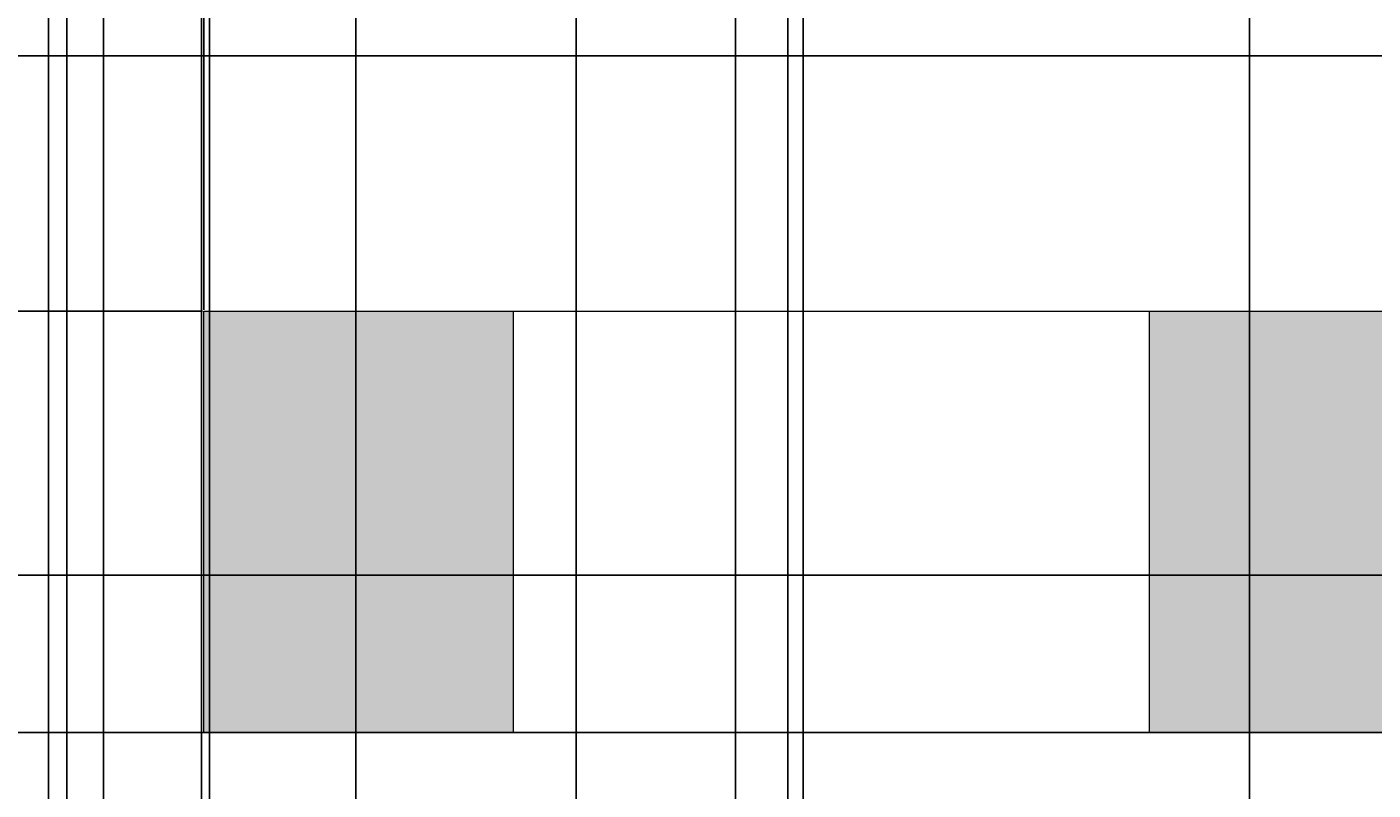
# Model space of a CAD drawing. Units: inches. Extents: x 818 to 1898, y 976 to 2364.
# Tile 68 of 96: x 1302 to 1372, y 1873 to 1913. Entities that reach past the tile are written whole.
import ezdxf

# ---------------------------------------------------------------- set-up
doc = ezdxf.new("R2010")
doc.units = ezdxf.units.IN
doc.header["$LTSCALE"] = 5
doc.header["$MEASUREMENT"] = 0
for name, color, linetype, lineweight in [('A-ANNO-DIMS', 2, 'Continuous', 18), ('A-FLOR-CASE', 8, 'Continuous', 18), ('A-FURN-PATT', 8, 'Continuous', 9)]:
    doc.layers.add(name, color=color, linetype=linetype, lineweight=lineweight)
doc.styles.get("Standard").update_dxf_attribs({"font": 'arial.ttf'})
doc.dimstyles.get("Standard").update_dxf_attribs({"dimtxt": 0.18, "dimasz": 0.18, "dimexe": 0.18, "dimexo": 0.0625, "dimgap": 0.09, "dimtad": 0, "dimtih": 1, "dimtoh": 1, "dimdec": 4, "dimzin": 0, "dimdsep": 46, "dimtxsty": 'Standard', "dimcen": 0.09, "dimadec": 0, "dimazin": 0, "dimtfac": 1, "dimtdec": 4, "dimtofl": 0, "dimtmove": 0, "dimatfit": 3, "dimfxl": 1, "dimtolj": 1, "dimtzin": 0, "dimarcsym": 0})

# ---------------------------------------------------------------- blocks, each defined once
blk = doc.blocks.new('*D61')
at = {"layer": 'A-ANNO-DIMS', "color": 0, "lineweight": -2, "ltscale": 5, "transparency": 16777216}
for p, q in [((1071.725, 1203.027), (1071.725, 2363.873)), ((1071.905, 2363.693), (1250.936, 2363.693)), ((1430.545, 2363.693), (1251.514, 2363.693)), ((1430.725, 1203.027), (1430.725, 2363.873))]:
    blk.add_line(p, q, dxfattribs=at)
at = {"layer": 'A-ANNO-DIMS', "color": 0, "ltscale": 5, "transparency": 16777216}
for points in [[(1071.905, 2363.723), (1071.905, 2363.663), (1071.725, 2363.693)], [(1430.545, 2363.723), (1430.545, 2363.663), (1430.725, 2363.693)]]:
    blk.add_solid(points, dxfattribs=at)
at = {"layer": 'Defpoints', "color": 0, "ltscale": 5, "transparency": 16777216}
for p in [(1430.725, 2363.693), (1071.725, 1202.964), (1430.725, 1202.964)]:
    blk.add_point(p, dxfattribs=at)
at = {"layer": 'A-ANNO-DIMS', "color": 0, "ltscale": 5, "transparency": 16777216, "insert": (1251.225, 2363.693), "char_height": 0.18, "attachment_point": 5}
blk.add_mtext('\\A1;359', dxfattribs=at)
blk = doc.blocks.new('*D64')
at = {"layer": 'A-ANNO-DIMS', "color": 0, "lineweight": -2, "ltscale": 5, "transparency": 16777216}
for p, q in [((1197.725, 1501.141), (1197.725, 2363.873)), ((1197.905, 2363.693), (1313.935, 2363.693)), ((1430.545, 2363.693), (1314.516, 2363.693)), ((1430.725, 1501.141), (1430.725, 2363.873))]:
    blk.add_line(p, q, dxfattribs=at)
at = {"layer": 'A-ANNO-DIMS', "color": 0, "ltscale": 5, "transparency": 16777216}
for points in [[(1197.905, 2363.723), (1197.905, 2363.663), (1197.725, 2363.693)], [(1430.545, 2363.723), (1430.545, 2363.663), (1430.725, 2363.693)]]:
    blk.add_solid(points, dxfattribs=at)
at = {"layer": 'Defpoints', "color": 0, "ltscale": 5, "transparency": 16777216}
for p in [(1430.725, 2363.693), (1197.725, 1501.078), (1430.725, 1501.078)]:
    blk.add_point(p, dxfattribs=at)
at = {"layer": 'A-ANNO-DIMS', "color": 0, "ltscale": 5, "transparency": 16777216, "insert": (1314.225, 2363.693), "char_height": 0.18, "attachment_point": 5}
blk.add_mtext('\\A1;233', dxfattribs=at)
blk = doc.blocks.new('*D74')
at = {"layer": 'A-ANNO-DIMS', "color": 0, "lineweight": -2, "ltscale": 5, "transparency": 16777216}
for p, q in [((1590.663, 1940.078), (818.026, 1940.078)), ((818.206, 1939.898), (818.206, 1925.76)), ((818.206, 1911.258), (818.206, 1925.396)), ((1590.663, 1911.078), (818.026, 1911.078))]:
    blk.add_line(p, q, dxfattribs=at)
at = {"layer": 'A-ANNO-DIMS', "color": 0, "ltscale": 5, "transparency": 16777216}
for points in [[(818.176, 1939.898), (818.236, 1939.898), (818.206, 1940.078)], [(818.176, 1911.258), (818.236, 1911.258), (818.206, 1911.078)]]:
    blk.add_solid(points, dxfattribs=at)
at = {"layer": 'Defpoints', "color": 0, "ltscale": 5, "transparency": 16777216}
for p in [(818.206, 1940.078), (1590.725, 1940.078), (1590.725, 1911.078)]:
    blk.add_point(p, dxfattribs=at)
at = {"layer": 'A-ANNO-DIMS', "color": 0, "ltscale": 5, "transparency": 16777216, "insert": (818.206, 1925.578), "char_height": 0.18, "attachment_point": 5}
blk.add_mtext('\\A1;29', dxfattribs=at)
blk = doc.blocks.new('*D85')
at = {"layer": 'A-ANNO-DIMS', "color": 0, "lineweight": -2, "ltscale": 5, "transparency": 16777216}
for p, q in [((1258.788, 2053.078), (1897.916, 2053.078)), ((1897.736, 2052.898), (1897.736, 1876.76)), ((1897.736, 1700.258), (1897.736, 1876.396)), ((1258.788, 1700.078), (1897.916, 1700.078))]:
    blk.add_line(p, q, dxfattribs=at)
at = {"layer": 'A-ANNO-DIMS', "color": 0, "ltscale": 5, "transparency": 16777216}
for points in [[(1897.706, 2052.898), (1897.766, 2052.898), (1897.736, 2053.078)], [(1897.706, 1700.258), (1897.766, 1700.258), (1897.736, 1700.078)]]:
    blk.add_solid(points, dxfattribs=at)
at = {"layer": 'Defpoints', "color": 0, "ltscale": 5, "transparency": 16777216}
for p in [(1258.725, 2053.078), (1897.736, 2053.078), (1258.725, 1700.078)]:
    blk.add_point(p, dxfattribs=at)
at = {"layer": 'A-ANNO-DIMS', "color": 0, "ltscale": 5, "transparency": 16777216, "insert": (1897.736, 1876.578), "char_height": 0.18, "attachment_point": 5}
blk.add_mtext('\\A1;353', dxfattribs=at)
blk = doc.blocks.new('*D97')
at = {"layer": 'A-ANNO-DIMS', "color": 0, "lineweight": -2, "ltscale": 5, "transparency": 16777216}
for p, q in [((1284.17, 1071.118), (1284.17, 2363.873)), ((1284.35, 2363.693), (1310.962, 2363.693)), ((1338.361, 2363.693), (1311.749, 2363.693)), ((1338.541, 1071.118), (1338.541, 2363.873))]:
    blk.add_line(p, q, dxfattribs=at)
at = {"layer": 'A-ANNO-DIMS', "color": 0, "ltscale": 5, "transparency": 16777216}
for points in [[(1284.35, 2363.723), (1284.35, 2363.663), (1284.17, 2363.693)], [(1338.361, 2363.723), (1338.361, 2363.663), (1338.541, 2363.693)]]:
    blk.add_solid(points, dxfattribs=at)
at = {"layer": 'Defpoints', "color": 0, "ltscale": 5, "transparency": 16777216}
for p in [(1338.541, 2363.693), (1284.17, 1071.055), (1338.541, 1071.055)]:
    blk.add_point(p, dxfattribs=at)
at = {"layer": 'A-ANNO-DIMS', "color": 0, "ltscale": 5, "transparency": 16777216, "insert": (1311.355, 2363.693), "char_height": 0.18, "attachment_point": 5}
blk.add_mtext('\\A1;54.37', dxfattribs=at)
blk = doc.blocks.new('*D98')
at = {"layer": 'A-ANNO-DIMS', "color": 0, "lineweight": -2, "ltscale": 5, "transparency": 16777216}
for p, q in [((1338.541, 1071.118), (1338.541, 2363.873)), ((1338.721, 2363.693), (1364.815, 2363.693)), ((1391.696, 2363.693), (1365.602, 2363.693)), ((1391.876, 1071.118), (1391.876, 2363.873))]:
    blk.add_line(p, q, dxfattribs=at)
at = {"layer": 'A-ANNO-DIMS', "color": 0, "ltscale": 5, "transparency": 16777216}
for points in [[(1338.721, 2363.723), (1338.721, 2363.663), (1338.541, 2363.693)], [(1391.696, 2363.723), (1391.696, 2363.663), (1391.876, 2363.693)]]:
    blk.add_solid(points, dxfattribs=at)
at = {"layer": 'Defpoints', "color": 0, "ltscale": 5, "transparency": 16777216}
for p in [(1391.876, 2363.693), (1338.541, 1071.055), (1391.876, 1071.055)]:
    blk.add_point(p, dxfattribs=at)
at = {"layer": 'A-ANNO-DIMS', "color": 0, "ltscale": 5, "transparency": 16777216, "insert": (1365.208, 2363.693), "char_height": 0.18, "attachment_point": 5}
blk.add_mtext('\\A1;53.33', dxfattribs=at)
blk = doc.blocks.new('*D121')
at = {"layer": 'A-ANNO-DIMS', "color": 0, "lineweight": -2, "ltscale": 5, "transparency": 16777216}
for p, q in [((1766.29, 1884.203), (818.026, 1884.203)), ((818.206, 1884.023), (818.206, 1841.142)), ((818.206, 1797.897), (818.206, 1840.778)), ((1766.29, 1797.717), (818.026, 1797.717))]:
    blk.add_line(p, q, dxfattribs=at)
at = {"layer": 'A-ANNO-DIMS', "color": 0, "ltscale": 5, "transparency": 16777216}
for points in [[(818.176, 1884.023), (818.236, 1884.023), (818.206, 1884.203)], [(818.176, 1797.897), (818.236, 1797.897), (818.206, 1797.717)]]:
    blk.add_solid(points, dxfattribs=at)
at = {"layer": 'Defpoints', "color": 0, "ltscale": 5, "transparency": 16777216}
for p in [(818.206, 1884.203), (1766.352, 1884.203), (1766.352, 1797.717)]:
    blk.add_point(p, dxfattribs=at)
at = {"layer": 'A-ANNO-DIMS', "color": 0, "ltscale": 5, "transparency": 16777216, "insert": (818.206, 1840.96), "char_height": 0.18, "attachment_point": 5}
blk.add_mtext('\\A1;86.49', dxfattribs=at)
blk = doc.blocks.new('*D162')
at = {"layer": 'A-ANNO-DIMS', "color": 0, "lineweight": -2, "ltscale": 5, "transparency": 16777216}
for p, q in [((1429.163, 1876.078), (818.026, 1876.078)), ((818.206, 1875.898), (818.206, 1871.76)), ((818.206, 1867.258), (818.206, 1871.396)), ((1429.163, 1867.078), (818.026, 1867.078))]:
    blk.add_line(p, q, dxfattribs=at)
at = {"layer": 'A-ANNO-DIMS', "color": 0, "ltscale": 5, "transparency": 16777216}
for points in [[(818.176, 1875.898), (818.236, 1875.898), (818.206, 1876.078)], [(818.176, 1867.258), (818.236, 1867.258), (818.206, 1867.078)]]:
    blk.add_solid(points, dxfattribs=at)
at = {"layer": 'Defpoints', "color": 0, "ltscale": 5, "transparency": 16777216}
for p in [(1429.225, 1876.078), (818.206, 1867.078), (1429.225, 1867.078)]:
    blk.add_point(p, dxfattribs=at)
at = {"layer": 'A-ANNO-DIMS', "color": 0, "ltscale": 5, "transparency": 16777216, "insert": (818.206, 1871.578), "char_height": 0.18, "attachment_point": 5}
blk.add_mtext('\\A1;9', dxfattribs=at)
blk = doc.blocks.new('*D165')
at = {"layer": 'A-ANNO-DIMS', "color": 0, "lineweight": -2, "ltscale": 5, "transparency": 16777216}
for p, q in [((1283.818, 1510.141), (1283.818, 2363.873)), ((1283.998, 2363.693), (1324.088, 2363.693)), ((1364.966, 2363.693), (1324.876, 2363.693)), ((1365.146, 1510.141), (1365.146, 2363.873))]:
    blk.add_line(p, q, dxfattribs=at)
at = {"layer": 'A-ANNO-DIMS', "color": 0, "ltscale": 5, "transparency": 16777216}
for points in [[(1283.998, 2363.723), (1283.998, 2363.663), (1283.818, 2363.693)], [(1364.966, 2363.723), (1364.966, 2363.663), (1365.146, 2363.693)]]:
    blk.add_solid(points, dxfattribs=at)
at = {"layer": 'Defpoints', "color": 0, "ltscale": 5, "transparency": 16777216}
for p in [(1365.146, 2363.693), (1283.818, 1510.078), (1365.146, 1510.078)]:
    blk.add_point(p, dxfattribs=at)
at = {"layer": 'A-ANNO-DIMS', "color": 0, "ltscale": 5, "transparency": 16777216, "insert": (1324.482, 2363.693), "char_height": 0.18, "attachment_point": 5}
blk.add_mtext('\\A1;81.33', dxfattribs=at)
blk = doc.blocks.new('*D206')
at = {"layer": 'A-ANNO-DIMS', "color": 0, "lineweight": -2, "ltscale": 5, "transparency": 16777216}
for p, q in [((1590.663, 1911.078), (818.026, 1911.078)), ((818.206, 1910.898), (818.206, 1893.76)), ((818.206, 1876.258), (818.206, 1893.396)), ((1590.663, 1876.078), (818.026, 1876.078))]:
    blk.add_line(p, q, dxfattribs=at)
at = {"layer": 'A-ANNO-DIMS', "color": 0, "ltscale": 5, "transparency": 16777216}
for points in [[(818.176, 1910.898), (818.236, 1910.898), (818.206, 1911.078)], [(818.176, 1876.258), (818.236, 1876.258), (818.206, 1876.078)]]:
    blk.add_solid(points, dxfattribs=at)
at = {"layer": 'Defpoints', "color": 0, "ltscale": 5, "transparency": 16777216}
for p in [(818.206, 1911.078), (1590.725, 1911.078), (1590.725, 1876.078)]:
    blk.add_point(p, dxfattribs=at)
at = {"layer": 'A-ANNO-DIMS', "color": 0, "ltscale": 5, "transparency": 16777216, "insert": (818.206, 1893.578), "char_height": 0.18, "attachment_point": 5}
blk.add_mtext('\\A1;35', dxfattribs=at)
blk = doc.blocks.new('*D215')
at = {"layer": 'A-ANNO-DIMS', "color": 0, "lineweight": -2, "ltscale": 5, "transparency": 16777216}
for p, q in [((1590.663, 1876.078), (818.026, 1876.078)), ((818.206, 1875.898), (818.206, 1781.76)), ((818.206, 1687.258), (818.206, 1781.396)), ((1511.663, 1687.078), (818.026, 1687.078))]:
    blk.add_line(p, q, dxfattribs=at)
at = {"layer": 'A-ANNO-DIMS', "color": 0, "ltscale": 5, "transparency": 16777216}
for points in [[(818.176, 1875.898), (818.236, 1875.898), (818.206, 1876.078)], [(818.176, 1687.258), (818.236, 1687.258), (818.206, 1687.078)]]:
    blk.add_solid(points, dxfattribs=at)
at = {"layer": 'Defpoints', "color": 0, "ltscale": 5, "transparency": 16777216}
for p in [(818.206, 1876.078), (1590.725, 1876.078), (1511.725, 1687.078)]:
    blk.add_point(p, dxfattribs=at)
at = {"layer": 'A-ANNO-DIMS', "color": 0, "ltscale": 5, "transparency": 16777216, "insert": (818.206, 1781.578), "char_height": 0.18, "attachment_point": 5}
blk.add_mtext('\\A1;189', dxfattribs=at)
blk = doc.blocks.new('*D231')
at = {"layer": 'A-ANNO-DIMS', "color": 0, "lineweight": -2, "ltscale": 5, "transparency": 16777216}
for p, q in [((1303.931, 1952.978), (1303.931, 975.663)), ((1402.518, 1952.978), (1402.518, 975.663)), ((1304.111, 975.843), (1352.831, 975.843)), ((1402.338, 975.843), (1353.619, 975.843))]:
    blk.add_line(p, q, dxfattribs=at)
at = {"layer": 'A-ANNO-DIMS', "color": 0, "ltscale": 5, "transparency": 16777216}
for points in [[(1304.111, 975.873), (1304.111, 975.813), (1303.931, 975.843)], [(1402.338, 975.873), (1402.338, 975.813), (1402.518, 975.843)]]:
    blk.add_solid(points, dxfattribs=at)
at = {"layer": 'Defpoints', "color": 0, "ltscale": 5, "transparency": 16777216}
for p in [(1303.931, 1953.041), (1402.518, 1953.041), (1402.518, 975.843)]:
    blk.add_point(p, dxfattribs=at)
at = {"layer": 'A-ANNO-DIMS', "color": 0, "ltscale": 5, "transparency": 16777216, "insert": (1353.225, 975.843), "char_height": 0.18, "attachment_point": 5}
blk.add_mtext('\\A1;98.59', dxfattribs=at)
blk = doc.blocks.new('*D233')
at = {"layer": 'A-ANNO-DIMS', "color": 0, "lineweight": -2, "ltscale": 5, "transparency": 16777216}
for p, q in [((1267.725, 2044.016), (1267.725, 975.663)), ((1303.931, 2008.329), (1303.931, 975.663)), ((1267.905, 975.843), (1285.365, 975.843)), ((1303.751, 975.843), (1286.292, 975.843))]:
    blk.add_line(p, q, dxfattribs=at)
at = {"layer": 'A-ANNO-DIMS', "color": 0, "ltscale": 5, "transparency": 16777216}
for points in [[(1267.905, 975.873), (1267.905, 975.813), (1267.725, 975.843)], [(1303.751, 975.873), (1303.751, 975.813), (1303.931, 975.843)]]:
    blk.add_solid(points, dxfattribs=at)
at = {"layer": 'Defpoints', "color": 0, "ltscale": 5, "transparency": 16777216}
for p in [(1267.725, 2044.078), (1303.931, 2008.392), (1303.931, 975.843)]:
    blk.add_point(p, dxfattribs=at)
at = {"layer": 'A-ANNO-DIMS', "color": 0, "ltscale": 5, "transparency": 16777216, "insert": (1285.828, 975.843), "char_height": 0.18, "attachment_point": 5}
blk.add_mtext('\\A1;36.206', dxfattribs=at)
blk = doc.blocks.new('*D236')
at = {"layer": 'A-ANNO-DIMS', "color": 0, "lineweight": -2, "ltscale": 5, "transparency": 16777216}
for p, q in [((1310.908, 2026.145), (1310.908, 975.663)), ((1342.045, 2026.145), (1342.045, 975.663)), ((1311.088, 975.843), (1326.083, 975.843)), ((1341.865, 975.843), (1326.87, 975.843))]:
    blk.add_line(p, q, dxfattribs=at)
at = {"layer": 'A-ANNO-DIMS', "color": 0, "ltscale": 5, "transparency": 16777216}
for points in [[(1311.088, 975.873), (1311.088, 975.813), (1310.908, 975.843)], [(1341.865, 975.873), (1341.865, 975.813), (1342.045, 975.843)]]:
    blk.add_solid(points, dxfattribs=at)
at = {"layer": 'Defpoints', "color": 0, "ltscale": 5, "transparency": 16777216}
for p in [(1310.908, 2026.207), (1342.045, 2026.207), (1342.045, 975.843)]:
    blk.add_point(p, dxfattribs=at)
at = {"layer": 'A-ANNO-DIMS', "color": 0, "ltscale": 5, "transparency": 16777216, "insert": (1326.476, 975.843), "char_height": 0.18, "attachment_point": 5}
blk.add_mtext('\\A1;31.14', dxfattribs=at)
blk = doc.blocks.new('*D252')
at = {"layer": 'A-ANNO-DIMS', "color": 0, "lineweight": -2, "ltscale": 5, "transparency": 16777216}
for p, q in [((1330.305, 2053.016), (1330.305, 975.663)), ((1388.031, 2053.016), (1388.031, 975.663)), ((1330.485, 975.843), (1358.775, 975.843)), ((1387.851, 975.843), (1359.562, 975.843))]:
    blk.add_line(p, q, dxfattribs=at)
at = {"layer": 'A-ANNO-DIMS', "color": 0, "ltscale": 5, "transparency": 16777216}
for points in [[(1330.485, 975.873), (1330.485, 975.813), (1330.305, 975.843)], [(1387.851, 975.873), (1387.851, 975.813), (1388.031, 975.843)]]:
    blk.add_solid(points, dxfattribs=at)
at = {"layer": 'Defpoints', "color": 0, "ltscale": 5, "transparency": 16777216}
for p in [(1330.305, 2053.078), (1388.031, 2053.078), (1388.031, 975.843)]:
    blk.add_point(p, dxfattribs=at)
at = {"layer": 'A-ANNO-DIMS', "color": 0, "ltscale": 5, "transparency": 16777216, "insert": (1359.168, 975.843), "char_height": 0.18, "attachment_point": 5}
blk.add_mtext('\\A1;57.73', dxfattribs=at)
blk = doc.blocks.new('*D254')
at = {"layer": 'A-ANNO-DIMS', "color": 0, "lineweight": -2, "ltscale": 5, "transparency": 16777216}
for p, q in [((1267.725, 2044.016), (1267.725, 975.663)), ((1330.305, 2044.016), (1330.305, 975.663)), ((1267.905, 975.843), (1298.621, 975.843)), ((1330.125, 975.843), (1299.409, 975.843))]:
    blk.add_line(p, q, dxfattribs=at)
at = {"layer": 'A-ANNO-DIMS', "color": 0, "ltscale": 5, "transparency": 16777216}
for points in [[(1267.905, 975.873), (1267.905, 975.813), (1267.725, 975.843)], [(1330.125, 975.873), (1330.125, 975.813), (1330.305, 975.843)]]:
    blk.add_solid(points, dxfattribs=at)
at = {"layer": 'Defpoints', "color": 0, "ltscale": 5, "transparency": 16777216}
for p in [(1267.725, 2044.078), (1330.305, 2044.078), (1330.305, 975.843)]:
    blk.add_point(p, dxfattribs=at)
at = {"layer": 'A-ANNO-DIMS', "color": 0, "ltscale": 5, "transparency": 16777216, "insert": (1299.015, 975.843), "char_height": 0.18, "attachment_point": 5}
blk.add_mtext('\\A1;62.58', dxfattribs=at)
blk = doc.blocks.new('*D269')
at = {"layer": 'A-ANNO-DIMS', "color": 0, "lineweight": -2, "ltscale": 5, "transparency": 16777216}
for p, q in [((1246.938, 1534.141), (1246.938, 2363.873)), ((1247.118, 2363.693), (1293.706, 2363.693)), ((1341.079, 2363.693), (1294.491, 2363.693)), ((1341.259, 1534.141), (1341.259, 2363.873))]:
    blk.add_line(p, q, dxfattribs=at)
at = {"layer": 'A-ANNO-DIMS', "color": 0, "ltscale": 5, "transparency": 16777216}
for points in [[(1247.118, 2363.723), (1247.118, 2363.663), (1246.938, 2363.693)], [(1341.079, 2363.723), (1341.079, 2363.663), (1341.259, 2363.693)]]:
    blk.add_solid(points, dxfattribs=at)
at = {"layer": 'Defpoints', "color": 0, "ltscale": 5, "transparency": 16777216}
for p in [(1341.259, 2363.693), (1246.938, 1534.078), (1341.259, 1534.078)]:
    blk.add_point(p, dxfattribs=at)
at = {"layer": 'A-ANNO-DIMS', "color": 0, "ltscale": 5, "transparency": 16777216, "insert": (1294.099, 2363.693), "char_height": 0.18, "attachment_point": 5}
blk.add_mtext('\\A1;94.32', dxfattribs=at)
blk = doc.blocks.new('*D274')
at = {"layer": 'A-ANNO-DIMS', "color": 0, "lineweight": -2, "ltscale": 5, "transparency": 16777216}
for p, q in [((1311.025, 1897.929), (1311.025, 2363.873)), ((1311.205, 2363.693), (1344.007, 2363.693)), ((1377.599, 2363.693), (1344.797, 2363.693)), ((1377.779, 1897.929), (1377.779, 2363.873))]:
    blk.add_line(p, q, dxfattribs=at)
at = {"layer": 'A-ANNO-DIMS', "color": 0, "ltscale": 5, "transparency": 16777216}
for points in [[(1311.205, 2363.723), (1311.205, 2363.663), (1311.025, 2363.693)], [(1377.599, 2363.723), (1377.599, 2363.663), (1377.779, 2363.693)]]:
    blk.add_solid(points, dxfattribs=at)
at = {"layer": 'Defpoints', "color": 0, "ltscale": 5, "transparency": 16777216}
for p in [(1377.779, 2363.693), (1311.025, 1897.866), (1377.779, 1897.866)]:
    blk.add_point(p, dxfattribs=at)
at = {"layer": 'A-ANNO-DIMS', "color": 0, "ltscale": 5, "transparency": 16777216, "insert": (1344.402, 2363.693), "char_height": 0.18, "attachment_point": 5}
blk.add_mtext('\\A1;66.75', dxfattribs=at)
blk = doc.blocks.new('*D286')
at = {"layer": 'A-ANNO-DIMS', "color": 0, "lineweight": -2, "ltscale": 5, "transparency": 16777216}
for p, q in [((1305.828, 1851.971), (1305.828, 2363.873)), ((1306.008, 2363.693), (1308.184, 2363.693)), ((1311.147, 2363.693), (1308.971, 2363.693)), ((1311.327, 1853.812), (1311.327, 2363.873))]:
    blk.add_line(p, q, dxfattribs=at)
at = {"layer": 'A-ANNO-DIMS', "color": 0, "ltscale": 5, "transparency": 16777216}
for points in [[(1306.008, 2363.723), (1306.008, 2363.663), (1305.828, 2363.693)], [(1311.147, 2363.723), (1311.147, 2363.663), (1311.327, 2363.693)]]:
    blk.add_solid(points, dxfattribs=at)
at = {"layer": 'Defpoints', "color": 0, "ltscale": 5, "transparency": 16777216}
for p in [(1305.828, 2363.693), (1311.327, 1853.75), (1305.828, 1851.908)]:
    blk.add_point(p, dxfattribs=at)
at = {"layer": 'A-ANNO-DIMS', "color": 0, "ltscale": 5, "transparency": 16777216, "insert": (1308.577, 2363.693), "char_height": 0.18, "attachment_point": 5}
blk.add_mtext('\\A1;5.499', dxfattribs=at)
blk = doc.blocks.new('*D287')
at = {"layer": 'A-ANNO-DIMS', "color": 0, "lineweight": -2, "ltscale": 5, "transparency": 16777216}
for p, q in [((1303.869, 1953.041), (818.026, 1953.041)), ((818.206, 1952.861), (818.206, 1925.635)), ((818.206, 1898.046), (818.206, 1925.272)), ((1310.963, 1897.866), (818.026, 1897.866))]:
    blk.add_line(p, q, dxfattribs=at)
at = {"layer": 'A-ANNO-DIMS', "color": 0, "ltscale": 5, "transparency": 16777216}
for points in [[(818.176, 1952.861), (818.236, 1952.861), (818.206, 1953.041)], [(818.176, 1898.046), (818.236, 1898.046), (818.206, 1897.866)]]:
    blk.add_solid(points, dxfattribs=at)
at = {"layer": 'Defpoints', "color": 0, "ltscale": 5, "transparency": 16777216}
for p in [(818.206, 1953.041), (1303.931, 1953.041), (1311.025, 1897.866)]:
    blk.add_point(p, dxfattribs=at)
at = {"layer": 'A-ANNO-DIMS', "color": 0, "ltscale": 5, "transparency": 16777216, "insert": (818.206, 1925.454), "char_height": 0.18, "attachment_point": 5}
blk.add_mtext('\\A1;55.17', dxfattribs=at)
blk = doc.blocks.new('*D290')
at = {"layer": 'A-ANNO-DIMS', "color": 0, "lineweight": -2, "ltscale": 5, "transparency": 16777216}
for p, q in [((1302.983, 1599.435), (1302.983, 2363.873)), ((1303.163, 2363.693), (1310.57, 2363.693)), ((1318.713, 2363.693), (1311.306, 2363.693)), ((1318.893, 1607.833), (1318.893, 2363.873))]:
    blk.add_line(p, q, dxfattribs=at)
at = {"layer": 'A-ANNO-DIMS', "color": 0, "ltscale": 5, "transparency": 16777216}
for points in [[(1303.163, 2363.723), (1303.163, 2363.663), (1302.983, 2363.693)], [(1318.713, 2363.723), (1318.713, 2363.663), (1318.893, 2363.693)]]:
    blk.add_solid(points, dxfattribs=at)
at = {"layer": 'Defpoints', "color": 0, "ltscale": 5, "transparency": 16777216}
for p in [(1318.893, 2363.693), (1318.893, 1607.771), (1302.983, 1599.372)]:
    blk.add_point(p, dxfattribs=at)
at = {"layer": 'A-ANNO-DIMS', "color": 0, "ltscale": 5, "transparency": 16777216, "insert": (1310.938, 2363.693), "char_height": 0.18, "attachment_point": 5}
blk.add_mtext('\\A1;15.91', dxfattribs=at)

msp = doc.modelspace()

# ---------------------------------------------------------------- hatches: boundary and pattern name
at = {"layer": 'A-FURN-PATT', "ltscale": 5}
h = msp.add_hatch(color=256, dxfattribs=at)
h.dxf.hatch_style = 1
h.paths.add_polyline_path([(1336.7936, 1953.0408), (1314.2595, 1953.0408), (1314.2595, 1941.0096), (1336.7936, 1941.0096)])
h.paths.add_polyline_path([(1338.9915, 1941.0096), (1336.7936, 1941.0096), (1336.7936, 1937.7177), (1314.2595, 1937.7177), (1314.2595, 1941.0096), (1310.9077, 1941.0096), (1310.9077, 1935.2252), (1338.9915, 1935.2252)])
h.paths.add_polyline_path([(1336.7936, 1941.0096), (1314.2595, 1941.0096), (1314.2595, 1937.7177), (1336.7936, 1937.7177)], flags=17)
h.paths.add_polyline_path([(1367.9307, 1959.6079), (1345.3966, 1959.6079), (1345.3966, 1941.0096), (1367.9307, 1941.0096)])
h.paths.add_polyline_path([(1398.8475, 1953.0408), (1376.3134, 1953.0408), (1376.3134, 1952.6393), (1390.1242, 1941.0096), (1398.8475, 1941.0096)])
h.paths.add_polyline_path([(1376.3134, 1952.6393), (1376.3134, 1941.0096), (1390.1242, 1941.0096)], flags=17)
h.paths.add_polyline_path([(1370.1286, 1941.0096), (1367.9307, 1941.0096), (1367.9307, 1937.7177), (1345.3966, 1937.7177), (1345.3966, 1941.0096), (1342.0448, 1941.0096), (1342.0448, 1935.2252), (1370.1286, 1935.2252)])
h.paths.add_polyline_path([(1367.9307, 1941.0096), (1345.3966, 1941.0096), (1345.3966, 1937.7177), (1367.9307, 1937.7177)], flags=17)
h.paths.add_polyline_path([(1390.1242, 1941.0096), (1376.3134, 1941.0096), (1376.3134, 1937.7177), (1394.0336, 1937.7177)], flags=17)
h.paths.add_polyline_path([(1394.0336, 1937.7177), (1376.3134, 1937.7177), (1376.3134, 1941.0096), (1372.9616, 1941.0096), (1372.9616, 1935.2252), (1396.9935, 1935.2252)])
h.paths.add_polyline_path([(1398.8475, 1941.0096), (1390.1242, 1941.0096), (1394.0336, 1937.7177), (1398.8475, 1937.7177)])
h.paths.add_polyline_path([(1401.0455, 1941.0096), (1398.8475, 1941.0096), (1398.8475, 1937.7177), (1394.0336, 1937.7177), (1396.9935, 1935.2252), (1401.0455, 1935.2252)])
h.paths.add_polyline_path([(1336.7936, 2020.4229), (1314.2595, 2020.4229), (1314.2595, 2008.3917), (1336.7936, 2008.3917)])
h.paths.add_polyline_path([(1336.7936, 2023.7149), (1314.2595, 2023.7149), (1314.2595, 2020.4229), (1336.7936, 2020.4229)], flags=17)
h.paths.add_polyline_path([(1338.9915, 2026.2074), (1310.9077, 2026.2074), (1310.9077, 2020.4229), (1314.2595, 2020.4229), (1314.2595, 2023.7149), (1336.7936, 2023.7149), (1336.7936, 2020.4229), (1338.9915, 2020.4229)])
h.paths.add_polyline_path([(1367.9307, 2023.7149), (1345.3966, 2023.7149), (1345.3966, 2020.4229), (1367.9307, 2020.4229)], flags=17)
h.paths.add_polyline_path([(1370.1286, 2026.2074), (1342.0448, 2026.2074), (1342.0448, 2020.4229), (1345.3966, 2020.4229), (1345.3966, 2023.7149), (1367.9307, 2023.7149), (1367.9307, 2020.4229), (1370.1286, 2020.4229)])
h.paths.add_polyline_path([(1367.9307, 2020.4229), (1345.3966, 2020.4229), (1345.3966, 2008.3917), (1367.9307, 2008.3917)])
h.paths.add_polyline_path([(1398.8475, 2020.4229), (1388.1824, 2020.4229), (1376.3134, 2010.4284), (1376.3134, 2008.3917), (1398.8475, 2008.3917)])
h.paths.add_polyline_path([(1392.0918, 2023.7149), (1376.3134, 2023.7149), (1376.3134, 2020.4229), (1388.1824, 2020.4229)], flags=17)
h.paths.add_polyline_path([(1388.1824, 2020.4229), (1376.3134, 2020.4229), (1376.3134, 2010.4284)], flags=17)
h.paths.add_polyline_path([(1395.0518, 2026.2074), (1372.9616, 2026.2074), (1372.9616, 2020.4229), (1376.3134, 2020.4229), (1376.3134, 2023.7149), (1392.0918, 2023.7149)])
h.paths.add_polyline_path([(1398.8475, 2023.7149), (1392.0918, 2023.7149), (1388.1824, 2020.4229), (1398.8475, 2020.4229)])
h.paths.add_polyline_path([(1401.0455, 2026.2074), (1395.0518, 2026.2074), (1392.0918, 2023.7149), (1398.8475, 2023.7149), (1398.8475, 2020.4229), (1401.0455, 2020.4229)])
h.paths.add_polyline_path([(1327.0339, 1897.8663), (1311.025, 1897.8663), (1311.025, 1876.0782), (1327.0339, 1876.0782)])
h.paths.add_polyline_path([(1377.7791, 1897.8663), (1359.9579, 1897.8663), (1359.9579, 1876.0782), (1377.7791, 1876.0782)])
h.paths.add_polyline_path([(1430.7251, 1541.0439), (1406.7252, 1541.0439), (1406.7252, 1525.9965), (1430.7251, 1525.9965)])
h.paths.add_polyline_path([(1430.7251, 1587.4164), (1406.7252, 1587.4164), (1406.7252, 1570.9187), (1430.7251, 1570.9187)])

# ---------------------------------------------------------------- linework, layer by layer
at = {"layer": 'A-FLOR-CASE'}
for p, q in [((1327.0339, 1897.8663), (1327.0339, 1876.0782)), ((1359.9579, 1897.8663), (1359.9579, 1876.0782)), ((1377.7791, 1876.0782), (1311.3271, 1876.0782)), ((1311.3271, 1876.0782), (1311.3271, 1867.0782))]:
    msp.add_line(p, q, dxfattribs=at)
msp.add_lwpolyline([(1377.7791, 1876.0782), (1311.025, 1876.0782), (1311.025, 1897.8663), (1377.7791, 1897.8663)], close=True, dxfattribs=at)

# ---------------------------------------------------------------- dimensions: what is measured, and where the dimension line sits
at = {"layer": 'A-ANNO-DIMS', "ltscale": 5}
for base, p1, p2, override, picture, middle in [((1430.7251, 2363.6929), (1071.7251, 1202.9642), (1430.7251, 1202.9642), {"dimdec": 0, "dimlfac": 1, "dimrnd": 0, "dimzin": 0, "dimdsep": 46, "dimlunit": 2}, '*D61', (1251.2251, 2363.6929)), ((1430.7251, 2363.6929), (1197.7251, 1501.0782), (1430.7251, 1501.0782), {"dimdec": 0, "dimlfac": 1, "dimrnd": 0, "dimzin": 0, "dimdsep": 46, "dimlunit": 2}, '*D64', (1314.2251, 2363.6929)), ((1341.2593, 2363.6929), (1246.9377, 1534.0782), (1341.2593, 1534.0782), {"dimdec": 2, "dimlfac": 1, "dimrnd": 0, "dimzin": 0, "dimdsep": 46, "dimlunit": 2}, '*D269', (1294.0985, 2363.6929)), ((1365.1463, 2363.6929), (1283.8183, 1510.0782), (1365.1463, 1510.0782), {"dimdec": 2, "dimlfac": 1, "dimrnd": 0, "dimzin": 0, "dimdsep": 46, "dimlunit": 2}, '*D165', (1324.4823, 2363.6929)), ((1338.5412, 2363.6929), (1284.1697, 1071.0552), (1338.5412, 1071.0552), {"dimdec": 2, "dimlfac": 1, "dimrnd": 0, "dimzin": 0, "dimdsep": 46, "dimlunit": 2}, '*D97', (1311.3554, 2363.6929)), ((1318.8931, 2363.6929), (1302.9835, 1599.3725), (1318.8931, 1607.7707), {"dimdec": 2, "dimlfac": 1, "dimrnd": 0, "dimzin": 0, "dimdsep": 46, "dimlunit": 2}, '*D290', (1310.9383, 2363.6929)), ((1305.8278, 2363.6929), (1311.3271, 1853.7496), (1305.8278, 1851.9081), {"dimdec": 3, "dimlfac": 1, "dimrnd": 0, "dimzin": 0, "dimdsep": 46, "dimlunit": 2}, '*D286', (1308.5774, 2363.6929)), ((1377.7791, 2363.6929), (1311.025, 1897.8663), (1377.7791, 1897.8663), {"dimdec": 2, "dimlfac": 1, "dimrnd": 0, "dimzin": 0, "dimdsep": 46, "dimlunit": 2}, '*D274', (1344.4021, 2363.6929)), ((1391.8757, 2363.6929), (1338.5412, 1071.0552), (1391.8757, 1071.0552), {"dimdec": 2, "dimlfac": 1, "dimrnd": 0, "dimzin": 0, "dimdsep": 46, "dimlunit": 2}, '*D98', (1365.2084, 2363.6929)), ((1388.0315, 975.8433), (1330.305, 2053.0782), (1388.0315, 2053.0782), {"dimdec": 2, "dimlfac": 1, "dimrnd": 0, "dimzin": 0, "dimdsep": 46, "dimlunit": 2}, '*D252', (1359.1682, 975.8433)), ((1303.9314, 975.8433), (1267.7251, 2044.0782), (1303.9314, 2008.3917), {"dimdec": 3, "dimlfac": 1, "dimrnd": 0, "dimzin": 0, "dimdsep": 46, "dimlunit": 2}, '*D233', (1285.8283, 975.8433)), ((1330.305, 975.8433), (1267.7251, 2044.0782), (1330.305, 2044.0782), {"dimdec": 2, "dimlfac": 1, "dimrnd": 0, "dimzin": 0, "dimdsep": 46, "dimlunit": 2}, '*D254', (1299.0151, 975.8433)), ((1342.0448, 975.8433), (1310.9077, 2026.2074), (1342.0448, 2026.2074), {"dimdec": 2, "dimlfac": 1, "dimrnd": 0, "dimzin": 0, "dimdsep": 46, "dimlunit": 2}, '*D236', (1326.4762, 975.8433)), ((1402.518, 975.8433), (1303.9314, 1953.0408), (1402.518, 1953.0408), {"dimdec": 2, "dimlfac": 1, "dimrnd": 0, "dimzin": 0, "dimdsep": 46, "dimlunit": 2}, '*D231', (1353.2247, 975.8433))]:
    dim = msp.add_linear_dim(base=base, p1=p1, p2=p2, dimstyle='Standard', override=override, dxfattribs=at)
    dim.commit()
    dim.dimension.update_dxf_attribs({"geometry": picture, "text_midpoint": middle})
for base, p1, p2, override, picture, middle in [((1897.736, 2053.0782), (1258.7251, 1700.0782), (1258.7251, 2053.0782), {"dimdec": 0, "dimlfac": 1, "dimrnd": 0, "dimzin": 0, "dimdsep": 46, "dimlunit": 2}, '*D85', (1897.736, 1876.5782)), ((818.2059, 1953.0408), (1311.025, 1897.8663), (1303.9314, 1953.0408), {"dimdec": 2, "dimlfac": 1, "dimrnd": 0, "dimzin": 0, "dimdsep": 46, "dimlunit": 2}, '*D287', (818.2059, 1925.4536)), ((818.2059, 1940.0782), (1590.7251, 1911.0782), (1590.7251, 1940.0782), {"dimdec": 0, "dimlfac": 1, "dimrnd": 0, "dimzin": 0, "dimdsep": 46, "dimlunit": 2}, '*D74', (818.2059, 1925.5782)), ((818.2059, 1911.0782), (1590.7251, 1876.0782), (1590.7251, 1911.0782), {"dimdec": 0, "dimlfac": 1, "dimrnd": 0, "dimzin": 0, "dimdsep": 46, "dimlunit": 2}, '*D206', (818.2059, 1893.5782)), ((818.2059, 1884.2031), (1766.3524, 1797.7165), (1766.3524, 1884.2031), {"dimdec": 2, "dimlfac": 1, "dimrnd": 0, "dimzin": 0, "dimdsep": 46, "dimlunit": 2}, '*D121', (818.2059, 1840.9598)), ((818.2059, 1876.0782), (1511.7251, 1687.0782), (1590.7251, 1876.0782), {"dimdec": 0, "dimlfac": 1, "dimrnd": 0, "dimzin": 0, "dimdsep": 46, "dimlunit": 2}, '*D215', (818.2059, 1781.5782)), ((818.2059, 1867.0782), (1429.2251, 1876.0782), (1429.2251, 1867.0782), {"dimdec": 0, "dimlfac": 1, "dimrnd": 0, "dimzin": 0, "dimdsep": 46, "dimlunit": 2}, '*D162', (818.2059, 1871.5782))]:
    dim = msp.add_linear_dim(base=base, p1=p1, p2=p2, angle=90, dimstyle='Standard', override=override, dxfattribs=at)
    dim.commit()
    dim.dimension.update_dxf_attribs({"geometry": picture, "text_midpoint": middle})

doc.saveas('drawing.dxf')
